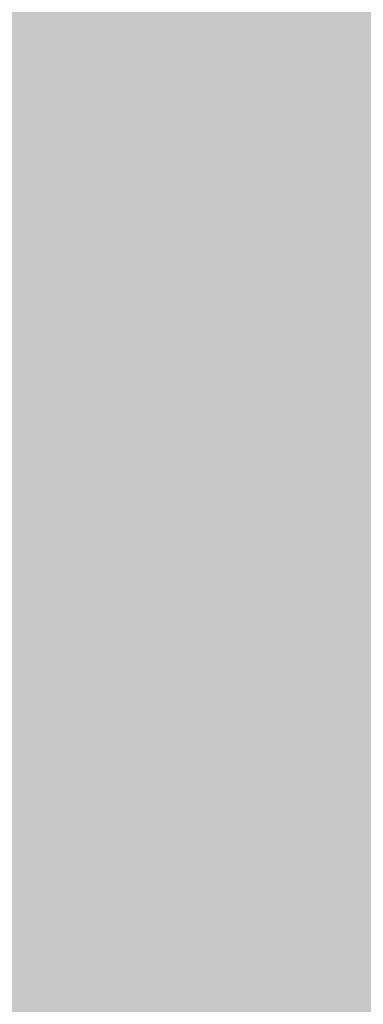
# Model space of a CAD drawing. Units: inches. Extents: x 2091 to 2899, y 967 to 2217.
# Tile 255 of 256: x 2246.06 to 2253.52, y 1131.25 to 1152.59. Entities that reach past the tile are written whole.
import ezdxf

# ---------------------------------------------------------------- set-up
doc = ezdxf.new("R2010")
doc.units = ezdxf.units.IN
doc.layers.add('A-ANNO-DIMS', color=2, linetype='Continuous', lineweight=18)
doc.layers.add('A-WALL-PATT', color=141, linetype='Continuous', lineweight=13, true_color=0xadddf7)
doc.layers.add('L-PLNT-PATT', color=114, linetype='Continuous', lineweight=13, true_color=0x139b48)
doc.styles.get("Standard").update_dxf_attribs({"font": 'arial.ttf'})
doc.dimstyles.new('ISO-25', dxfattribs={"dimtxt": 4, "dimasz": 4, "dimexe": 1.25, "dimexo": 0.625, "dimtad": 1, "dimdec": 0, "dimlunit": 3, "dimtxsty": 'Standard', "dimcen": 2.5, "dimadec": 0, "dimazin": 0, "dimtfac": 1, "dimtdec": 0, "dimtmove": 0, "dimatfit": 3, "dimfxl": 1, "dimarcsym": 0})

# ---------------------------------------------------------------- blocks, each defined once
blk = doc.blocks.new('*D71')
at = {"layer": 'A-ANNO-DIMS', "color": 0, "lineweight": -2, "transparency": 16777216}
for p, q in [((2212.144, 1351.294), (2212.144, 969.464)), ((2452.144, 1351.294), (2452.144, 969.464)), ((2216.144, 970.714), (2448.144, 970.714))]:
    blk.add_line(p, q, dxfattribs=at)
at = {"layer": 'A-ANNO-DIMS', "color": 0, "transparency": 16777216}
for points in [[(2216.144, 971.381), (2216.144, 970.048), (2212.144, 970.714)], [(2448.144, 971.381), (2448.144, 970.048), (2452.144, 970.714)]]:
    blk.add_solid(points, dxfattribs=at)
at = {"layer": 'Defpoints', "color": 0, "transparency": 16777216}
for p in [(2212.144, 1351.919), (2452.144, 1351.919), (2452.144, 970.714)]:
    blk.add_point(p, dxfattribs=at)
at = {"layer": 'A-ANNO-DIMS', "color": 0, "transparency": 16777216, "insert": (2332.144, 973.382), "char_height": 4, "attachment_point": 5}
blk.add_mtext('20\'-0"', dxfattribs=at)
blk = doc.blocks.new('*D75')
at = {"layer": 'A-ANNO-DIMS', "color": 0, "lineweight": -2, "transparency": 16777216}
for p, q in [((2212.144, 1274.794), (2212.144, 969.464)), ((2308.144, 1274.794), (2308.144, 969.464)), ((2216.144, 970.714), (2304.144, 970.714))]:
    blk.add_line(p, q, dxfattribs=at)
at = {"layer": 'A-ANNO-DIMS', "color": 0, "transparency": 16777216}
for points in [[(2216.144, 971.381), (2216.144, 970.048), (2212.144, 970.714)], [(2304.144, 971.381), (2304.144, 970.048), (2308.144, 970.714)]]:
    blk.add_solid(points, dxfattribs=at)
at = {"layer": 'Defpoints', "color": 0, "transparency": 16777216}
for p in [(2212.144, 1275.419), (2308.144, 1275.419), (2308.144, 970.714)]:
    blk.add_point(p, dxfattribs=at)
at = {"layer": 'A-ANNO-DIMS', "color": 0, "transparency": 16777216, "insert": (2260.144, 973.382), "char_height": 4, "attachment_point": 5}
blk.add_mtext('8\'-0"', dxfattribs=at)

msp = doc.modelspace()

# ---------------------------------------------------------------- hatches: boundary and pattern name
at = {"layer": 'A-WALL-PATT'}
h = msp.add_hatch(color=256, dxfattribs=at)
h.dxf.hatch_style = 1
h.paths.add_polyline_path([(2803.144, 2050.919), (2203.144, 2050.919), (2203.144, 1090.919), (2803.144, 1090.919)])
h.paths.add_polyline_path([(2635.799, 1147.54), (2674.524, 1147.54, 0.376086), (2678.53, 1152.88), (2678.53, 1159.556, 0.333335), (2674.524, 1163.562), (2674.524, 1163.562), (2674.524, 1192.934), (2635.806, 1192.934), (2597.088, 1192.934), (2597.088, 1163.562, 0.333335), (2593.082, 1159.556), (2593.082, 1152.88, 0.376086), (2597.088, 1147.54)], flags=0)
h.paths.add_polyline_path([(2436.01, 1278.241, 0.000483), (2435.953, 1278.215, -0.001328), (2435.936, 1278.112, -0.001711), (2436.116, 1278.041, 0.002185)], flags=0)
h.paths.add_polyline_path([(2794.144, 1143.419), (2794.144, 1347.419), (2543.37, 1347.419), (2543.37, 1351.919), (2794.144, 1351.919), (2794.144, 1392.714), (2793.947, 1392.714), (2793.947, 1473.537), (2794.144, 1473.537), (2794.144, 1531.919), (2650.144, 1531.919), (2650.144, 1536.419), (2794.144, 1536.419), (2794.144, 1692.419), (2609.376, 1692.419), (2609.376, 1644.419), (2604.876, 1644.419), (2604.876, 1744.919), (2609.376, 1744.919), (2609.376, 1696.919), (2794.144, 1696.919), (2794.144, 1780.919), (2609.644, 1780.919), (2493.876, 1780.919), (2493.876, 1785.419), (2609.644, 1785.419), (2794.144, 1785.419), (2794.144, 1847.939), (2793.951, 1847.939), (2793.951, 1928.762), (2794.144, 1928.762), (2794.144, 1941.419), (2614.144, 1941.419), (2614.144, 1821.419), (2609.644, 1821.419), (2609.644, 1941.419), (2392.144, 1941.419), (2392.144, 1819.919), (2387.644, 1819.919), (2387.644, 1941.419), (2212.144, 1941.419), (2212.144, 1783.919), (2392.144, 1783.919), (2392.144, 1780.919), (2212.144, 1780.919), (2212.144, 1629.419), (2387.644, 1629.419), (2387.644, 1744.919), (2392.144, 1744.919), (2392.144, 1627.919), (2317.144, 1627.919), (2317.144, 1551.419), (2317.144, 1536.419), (2459.384, 1536.419), (2459.384, 1602.396), (2463.884, 1602.396), (2463.884, 1531.919), (2456.644, 1531.919), (2456.644, 1529.919), (2452.144, 1529.919), (2452.144, 1531.919), (2312.644, 1531.919), (2312.644, 1551.419), (2306.144, 1551.419), (2306.144, 1555.919), (2308.144, 1555.919), (2308.144, 1551.419), (2312.644, 1551.419), (2312.644, 1627.919), (2212.144, 1627.919), (2212.144, 1555.919), (2270.144, 1555.919), (2270.144, 1551.419), (2212.144, 1551.419), (2212.144, 1351.919), (2272.144, 1351.919), (2272.144, 1347.419), (2212.144, 1347.419), (2212.144, 1275.419), (2308.144, 1275.419), (2308.144, 1351.919), (2452.144, 1351.919), (2452.144, 1493.919), (2456.644, 1493.919), (2456.644, 1347.419), (2312.644, 1347.419), (2312.644, 1270.919), (2212.144, 1270.919), (2212.144, 1099.919), (2281.238, 1099.919), (2282.871, 1110.914), (2282.008, 1116.997), (2278.558, 1121.42), (2268.206, 1128.056), (2272.088, 1128.056), (2273.813, 1131.927), (2279.42, 1134.692), (2285.028, 1135.245), (2287.616, 1137.457), (2288.047, 1138.01), (2289.341, 1140.775), (2291.067, 1139.669), (2292.361, 1135.245), (2295.38, 1136.904), (2296.243, 1135.798), (2297.105, 1133.033), (2300.125, 1138.01), (2303.144, 1138.01), (2304.438, 1135.798), (2303.144, 1133.586), (2306.595, 1134.692), (2307.889, 1133.033), (2310.908, 1135.245), (2313.927, 1134.139), (2315.627, 1132.427), (2308.32, 1117.55), (2290.204, 1109.808), (2288.91, 1103.172), (2289.272, 1099.919), (2434.918, 1099.919), (2431.593, 1124.788), (2429.93, 1169.553), (2430.927, 1240.52), (2435.659, 1238.186), (2437.135, 1196.554), (2438.798, 1143.973), (2442.678, 1111.998), (2446.558, 1099.919), (2794.144, 1099.919), (2794.144, 1138.919), (2548.032, 1138.919), (2548.032, 1143.419), (2548.032, 1148.819), (2546.668, 1148.032), (2528.686, 1179.179, 0.256256), (2512.032, 1148.819), (2512.032, 1143.419), (2512.032, 1138.919), (2507.532, 1138.919), (2507.532, 1143.419), (2507.532, 1148.819, 0.256256), (2490.879, 1179.179), (2472.896, 1148.032), (2471.532, 1148.819), (2471.532, 1143.419), (2467.032, 1143.419), (2467.032, 1269.946, 0.039061), (2460.91, 1273.58), (2467.032, 1273.58), (2467.032, 1286.325, 0.014511), (2465.216, 1286.762), (2467.032, 1287.053), (2467.032, 1323.419), (2471.532, 1323.419), (2471.532, 1148.819), (2489.532, 1179.996), (2490.896, 1179.208), (2490.879, 1179.179, -0.256256), (2507.532, 1148.819), (2507.532, 1143.419), (2512.032, 1143.419), (2512.032, 1148.819, -0.256256), (2528.686, 1179.179), (2528.668, 1179.208), (2530.032, 1179.996), (2548.032, 1148.819), (2548.032, 1143.419)], flags=16)
h.paths.add_polyline_path([(2607.769, 1200.945), (2607.769, 1265.031), (2597.088, 1281.052), (2619.785, 1281.052), (2627.795, 1337.127), (2635.799, 1337.127), (2643.817, 1337.127), (2651.827, 1281.052), (2674.524, 1281.052), (2663.843, 1265.031), (2663.843, 1200.945), (2635.806, 1200.945)], flags=0)
edge = h.paths.add_edge_path(flags=0)
edge.add_ellipse((13303.896, 1272.999), major_axis=(-10595.313, 0), ratio=0.84230387, start_angle=0.6282372, end_angle=0.6465541, ccw=False)
edge.add_ellipse((2711.7, 1156.853), major_axis=(2.22, 0), ratio=0.842304, start_angle=111.5352, end_angle=180.6282, ccw=False)
edge.add_ellipse((13303.156, 1272.999), major_axis=(-10593.026, 0), ratio=0.84230387, start_angle=0.5282715, end_angle=0.6465541, ccw=False)
edge.add_line((2710.765, 1175.333), (2710.13, 1175.333))
edge.add_ellipse((2710.13, 1176.58), major_axis=(1.48, 0), ratio=0.842304, start_angle=180, end_angle=270, ccw=False)
edge.add_line((2708.65, 1176.58), (2708.65, 1200.783))
edge.add_ellipse((2710.13, 1200.783), major_axis=(1.48, 0), ratio=0.842304, start_angle=90, end_angle=180, ccw=False)
edge.add_line((2710.13, 1202.029), (2710.465, 1202.029))
edge.add_ellipse((13303.156, 1272.999), major_axis=(-10593.026, 0), ratio=0.84230387, start_angle=-0.0902291, end_angle=0.3838668, ccw=False)
edge.add_ellipse((2710.13, 1290.927), major_axis=(-1.48, 0), ratio=0.842304, start_angle=0, end_angle=90, ccw=False)
edge.add_line((2708.65, 1290.927), (2708.65, 1315.13))
edge.add_ellipse((2710.13, 1315.13), major_axis=(-1.48, 0), ratio=0.842304, start_angle=-90, end_angle=0, ccw=False)
edge.add_line((2710.13, 1316.377), (2710.706, 1316.377))
edge.add_ellipse((3238.402, 1296.29), major_axis=(528.234, 0), ratio=0.8423039, start_angle=176.34957, end_angle=177.82005, ccw=False)
edge.add_ellipse((2775.063, 1071.451), major_axis=(313.308, 0), ratio=0.8423039, start_angle=102.12597, end_angle=103.78053, ccw=False)
edge.add_ellipse((2775.063, 1078.306), major_axis=(-305.303, 0), ratio=0.8423039, start_angle=-79.79046, end_angle=-77.55537, ccw=False)
edge.add_ellipse((2695.142, 1541.975), major_axis=(-250.96, 0), ratio=0.8423039, start_angle=99.25657, end_angle=102.55493)
edge.add_line((2741.41, 1334.214), (2747.133, 1337.378))
edge.add_ellipse((2747.539, 1336.857), major_axis=(-0.74, 0), ratio=0.842304, start_angle=270, end_angle=307.9331, ccw=False)
edge.add_ellipse((2747.539, 1336.857), major_axis=(-0.74, 0), ratio=0.842304, start_angle=232.0669, end_angle=270, ccw=False)
edge.add_line((2747.945, 1337.378), (2753.667, 1334.214))
edge.add_ellipse((2799.935, 1541.975), major_axis=(250.96, 0), ratio=0.8423039, start_angle=257.44507, end_angle=260.74343)
edge.add_ellipse((2720.014, 1078.306), major_axis=(305.303, 0), ratio=0.8423039, start_angle=77.55537, end_angle=79.79046, ccw=False)
edge.add_ellipse((2720.014, 1071.451), major_axis=(-313.308, 0), ratio=0.8423039, start_angle=256.21947, end_angle=257.87403, ccw=False)
edge.add_ellipse((2256.676, 1296.29), major_axis=(-528.234, 0), ratio=0.8423039, start_angle=182.17995, end_angle=183.65043, ccw=False)
edge.add_line((2784.371, 1316.377), (2784.947, 1316.377))
edge.add_ellipse((2784.947, 1315.13), major_axis=(1.48, 0), ratio=0.842304, start_angle=0, end_angle=90, ccw=False)
edge.add_line((2786.427, 1315.13), (2786.427, 1290.927))
edge.add_ellipse((2784.947, 1290.927), major_axis=(1.48, 0), ratio=0.842304, start_angle=270, end_angle=360, ccw=False)
edge.add_ellipse((-7808.079, 1272.999), major_axis=(10593.026, 0), ratio=0.84230387, start_angle=-0.3838668, end_angle=0.0902291, ccw=False)
edge.add_line((2784.612, 1202.029), (2784.947, 1202.029))
edge.add_ellipse((2784.947, 1200.783), major_axis=(1.48, 0), ratio=0.842304, start_angle=0, end_angle=90, ccw=False)
edge.add_line((2786.427, 1200.783), (2786.427, 1176.58))
edge.add_ellipse((2784.947, 1176.58), major_axis=(-1.48, 0), ratio=0.842304, start_angle=90, end_angle=180, ccw=False)
edge.add_line((2784.947, 1175.333), (2784.313, 1175.333))
edge.add_ellipse((-7808.079, 1272.999), major_axis=(10593.026, 0), ratio=0.84230387, start_angle=-0.6186432, end_angle=-0.5282715, ccw=False)
edge.add_ellipse((2783.377, 1156.853), major_axis=(-2.22, 0), ratio=0.842304, start_angle=179.3718, end_angle=248.4648, ccw=False)
edge.add_ellipse((-7808.819, 1272.999), major_axis=(-10595.313, 0), ratio=0.842303866, start_angle=179.3534459, end_angle=179.3717628, ccw=False)
edge.add_ellipse((2780.297, 1153.501), major_axis=(-5.246, 0), ratio=0.842304, start_angle=90, end_angle=179.3534, ccw=False)
edge.add_line((2780.297, 1149.082), (2714.78, 1149.082))
edge.add_ellipse((2714.78, 1153.501), major_axis=(5.246, 0), ratio=0.842304, start_angle=180.6466, end_angle=270, ccw=False)
edge = h.paths.add_edge_path(flags=0)
edge.add_line((2718.187, 1151.008), (2718.187, 1170.472))
edge.add_ellipse((2721.147, 1170.472), major_axis=(-2.96, 0), ratio=0.842304, start_angle=-90, end_angle=0, ccw=False)
edge.add_line((2721.147, 1172.965), (2773.93, 1172.965))
edge.add_ellipse((2773.93, 1170.472), major_axis=(-2.96, 0), ratio=0.842304, start_angle=180, end_angle=270, ccw=False)
edge.add_line((2776.89, 1170.472), (2776.89, 1151.008))
edge.add_line((2776.89, 1151.008), (2718.187, 1151.008))
edge = h.paths.add_edge_path(flags=0)
edge.add_line((2718.187, 1180.234), (2718.187, 1199.058))
edge.add_ellipse((2747.539, 1320.399), major_axis=(147.018, 0), ratio=0.8423039, start_angle=256.40187, end_angle=283.59813)
edge.add_line((2776.89, 1199.058), (2776.89, 1180.234))
edge.add_ellipse((2747.539, 1301.575), major_axis=(147.018, 0), ratio=0.8423039, start_angle=256.40187, end_angle=283.59813, ccw=False)
edge = h.paths.add_edge_path(flags=0)
edge.add_ellipse((13303.156, 1272.999), major_axis=(-10591.546, 0), ratio=0.84230387, start_angle=0.0555943, end_angle=0.3777642, ccw=False)
edge.add_line((2711.617, 1262.722), (2715.667, 1249.495))
edge.add_ellipse((6413.892, 1241.692), major_axis=(-3698.236, 0), ratio=0.84230387, start_angle=-0.120897, end_angle=0.364076)
edge.add_line((2715.761, 1218.192), (2711.934, 1203.167))
edge = h.paths.add_edge_path(flags=0)
edge.add_line((2718.187, 1251.075), (2716.002, 1267.45))
edge.add_ellipse((2742.151, 1202.19), major_axis=(81.773, 0), ratio=0.842304, start_angle=94.27742, end_angle=111.83495, ccw=False)
edge.add_line((2737.01, 1270.931), (2758.067, 1270.931))
edge.add_ellipse((2752.926, 1202.19), major_axis=(81.773, 0), ratio=0.842304, start_angle=68.16505, end_angle=85.72258, ccw=False)
edge.add_line((2779.075, 1267.45), (2776.89, 1251.075))
edge.add_ellipse((2750.338, 1187.885), major_axis=(79.58, 0), ratio=0.842304, start_angle=67.20809, end_angle=85.12993)
edge.add_line((2756.035, 1254.744), (2739.043, 1254.744))
edge.add_ellipse((2744.739, 1187.885), major_axis=(79.58, 0), ratio=0.842304, start_angle=94.87007, end_angle=112.79191)
edge = h.paths.add_edge_path(flags=0)
edge.add_line((2783.143, 1203.167), (2779.316, 1218.192))
edge.add_ellipse((-918.815, 1241.692), major_axis=(3698.236, 0), ratio=0.84230387, start_angle=-0.364076, end_angle=0.120897)
edge.add_line((2779.41, 1249.495), (2783.46, 1262.722))
edge.add_ellipse((-7808.079, 1272.999), major_axis=(-10591.546, 0), ratio=0.84230387, start_angle=179.6222358, end_angle=179.9444057, ccw=False)
edge = h.paths.add_edge_path(flags=0)
edge.add_ellipse((2734.201, 1286.69), major_axis=(-0.357, 6.34), ratio=0.603834, start_angle=89.002, end_angle=253.6574, ccw=False)
edge.add_line((2730.369, 1286.542), (2730.369, 1301.352))
edge.add_line((2730.369, 1301.352), (2735.913, 1305.215))
edge.add_ellipse((2736.385, 1304.735), major_axis=(0.74, 0), ratio=0.842304, start_angle=90, end_angle=134.4802, ccw=False)
edge.add_line((2736.385, 1305.358), (2738.033, 1305.358))
edge.add_line((2738.033, 1305.358), (2738.033, 1307.708))
edge.add_ellipse((2794.202, 1307.708), major_axis=(56.169, 0), ratio=0.842304, start_angle=150.5614, end_angle=180, ccw=False)
edge.add_ellipse((2700.876, 1307.708), major_axis=(-56.169, 0), ratio=0.842304, start_angle=180, end_angle=209.4386, ccw=False)
edge.add_line((2757.044, 1307.708), (2757.044, 1305.358))
edge.add_line((2757.044, 1305.358), (2758.692, 1305.358))
edge.add_ellipse((2758.692, 1304.735), major_axis=(-0.74, 0), ratio=0.842304, start_angle=225.5198, end_angle=270, ccw=False)
edge.add_line((2759.164, 1305.215), (2764.708, 1301.352))
edge.add_line((2764.708, 1301.352), (2764.708, 1286.542))
edge.add_ellipse((2760.876, 1286.69), major_axis=(0.357, 6.34), ratio=0.603834, start_angle=106.3426, end_angle=270.998, ccw=False)
edge.add_line((2757.044, 1285.797), (2757.044, 1307.708))
edge.add_ellipse((2700.876, 1307.708), major_axis=(-56.169, 0), ratio=0.842304, start_angle=180, end_angle=209.4386)
edge.add_ellipse((2794.202, 1307.708), major_axis=(56.169, 0), ratio=0.842304, start_angle=150.5614, end_angle=180)
edge.add_line((2738.033, 1307.708), (2738.033, 1285.797))
h.paths.add_polyline_path([(2417.812, 1104.45), (2413.492, 1102.53), (2410.612, 1103.97), (2409.172, 1106.37), (2407.252, 1107.33), (2406.292, 1109.73), (2405.332, 1114.05), (2405.332, 1117.89), (2406.292, 1120.13), (2407.252, 1119.81), (2408.848, 1118.328), (2410.174, 1119.424), (2410.211, 1120.406), (2411.041, 1121.419), (2410.699, 1119.859), (2410.174, 1119.424), (2410.088, 1117.176), (2411.133, 1116.206), (2413.972, 1119.33), (2416.852, 1120.77), (2416.87, 1120.799), (2417.035, 1119.405), (2417.896, 1118.143), (2418.292, 1118.37), (2419.544, 1120.039), (2419.361, 1118.387), (2419.032, 1119.356), (2418.399, 1118.512), (2419.252, 1114.53), (2418.794, 1107.199)], flags=0)
h.paths.add_polyline_path([(2508.87, 1347.419), (2508.37, 1347.419), (2508.37, 1351.919), (2508.87, 1351.919)], flags=0)
h.paths.add_polyline_path([(2473.37, 1347.419), (2472.37, 1347.419), (2467.87, 1347.419), (2467.87, 1455.419), (2472.37, 1455.419), (2472.37, 1352.419), (2473.37, 1352.419)], flags=0)
h.paths.add_polyline_path([(2352.106, 1217.446), (2349.226, 1218.886), (2347.786, 1221.286), (2345.866, 1222.246), (2344.906, 1224.646), (2343.946, 1228.966), (2343.946, 1232.806), (2344.906, 1235.046), (2345.866, 1234.726), (2347.462, 1233.244), (2348.788, 1234.341), (2348.825, 1235.322), (2349.655, 1236.336), (2349.313, 1234.775), (2348.788, 1234.341), (2348.702, 1232.093), (2349.747, 1231.123), (2352.586, 1234.246), (2355.466, 1235.686), (2355.484, 1235.715), (2355.649, 1234.322), (2356.51, 1233.06), (2356.906, 1233.286), (2358.158, 1234.956), (2357.975, 1233.304), (2357.646, 1234.273), (2357.013, 1233.428), (2357.866, 1229.446), (2357.408, 1222.115), (2356.426, 1219.366)], flags=0)
h.paths.add_polyline_path([(2348.297, 1112.224), (2347.014, 1112.31), (2345.53, 1114.127), (2345.732, 1115.858), (2346.812, 1116.982), (2346.812, 1114.646), (2345.867, 1114.214), (2346.88, 1114.3)], flags=0)
h.paths.add_polyline_path([(2347.014, 1110.926), (2346.272, 1110.493), (2346.61, 1111.186)], flags=0)
h.paths.add_polyline_path([(2345.867, 1118.194), (2345.53, 1117.329), (2343.708, 1118.021), (2344.383, 1118.626)], flags=0)
h.paths.add_polyline_path([(2346.677, 1109.282), (2346.07, 1108.071), (2345.867, 1110.061)], flags=0)
h.paths.add_polyline_path([(2345.057, 1119.751), (2343.64, 1119.751), (2343.978, 1121.135)], flags=0)
h.paths.add_polyline_path([(2345.26, 1116.55), (2345.125, 1115.858), (2344.922, 1115.685), (2344.72, 1116.377)], flags=0)
h.paths.add_polyline_path([(2345.665, 1112.31), (2345.462, 1111.532), (2344.045, 1111.964), (2344.652, 1112.57)], flags=0)
h.paths.add_polyline_path([(2345.192, 1113.349), (2344.45, 1113.868), (2344.72, 1114.387)], flags=0)
h.paths.add_polyline_path([(2344.652, 1116.809), (2344.18, 1115.685), (2344.652, 1115.339), (2343.91, 1114.906), (2343.033, 1115.944), (2343.64, 1116.463)], flags=0)
h.paths.add_polyline_path([(2345.867, 1106.686), (2344.99, 1105.562), (2344.517, 1106.6)], flags=0)
h.paths.add_polyline_path([(2344.855, 1110.061), (2344.517, 1109.282), (2344.113, 1109.715)], flags=0)
h.paths.add_polyline_path([(2344.045, 1113.522), (2343.438, 1113.089), (2342.763, 1113.954)], flags=0)
h.paths.add_polyline_path([(2344.315, 1111.012), (2342.965, 1110.32), (2342.965, 1111.099)], flags=0)
h.paths.add_polyline_path([(2345.125, 1104.697), (2344.585, 1103.745), (2344.45, 1104.264)], flags=0)
h.paths.add_polyline_path([(2342.83, 1121.222), (2341.75, 1120.53), (2340.536, 1121.049), (2340.131, 1121.828), (2340.671, 1122.952), (2341.143, 1121.828), (2341.615, 1122.001)], flags=0)
h.paths.add_polyline_path([(2342.965, 1119.751), (2343.033, 1118.453), (2342.088, 1118.021), (2342.02, 1119.491)], flags=0)
h.paths.add_polyline_path([(2342.695, 1116.896), (2341.953, 1116.636), (2342.02, 1117.329)], flags=0)
h.paths.add_polyline_path([(2343.033, 1112.224), (2342.02, 1111.791), (2341.548, 1112.224), (2342.358, 1113.349)], flags=0)
h.paths.add_polyline_path([(2343.775, 1104.437), (2342.628, 1102.88), (2342.695, 1104.61), (2343.438, 1105.129)], flags=0)
h.paths.add_polyline_path([(2342.02, 1115.079), (2340.806, 1115.512), (2340.941, 1116.377)], flags=0)
h.paths.add_polyline_path([(2341.481, 1120.097), (2341.481, 1119.405), (2341.076, 1119.578), (2341.143, 1120.097)], flags=0)
h.paths.add_polyline_path([(2341.818, 1114.473), (2340.941, 1113.089), (2340.806, 1114.56)], flags=0)
h.paths.add_polyline_path([(2341.143, 1118.54), (2340.941, 1116.982), (2339.051, 1117.675), (2339.051, 1118.626)], flags=0)
h.paths.add_polyline_path([(2342.695, 1101.668), (2341.953, 1101.841), (2342.56, 1102.361)], flags=0)
h.paths.add_polyline_path([(2340.333, 1119.665), (2338.444, 1119.578), (2337.904, 1120.357), (2339.658, 1120.616)], flags=0)
h.paths.add_polyline_path([(2340.333, 1115.339), (2340.063, 1113.695), (2339.388, 1115.339)], flags=0)
h.paths.add_polyline_path([(2341.818, 1103.831), (2341.548, 1102.88), (2341.143, 1103.658)], flags=0)
h.paths.add_polyline_path([(2339.051, 1122.866), (2337.296, 1121.828), (2337.094, 1123.125), (2337.769, 1123.818)], flags=0)
h.paths.add_polyline_path([(2339.118, 1121.741), (2338.848, 1121.222), (2338.174, 1121.049), (2338.376, 1121.568)], flags=0)
h.paths.add_polyline_path([(2339.186, 1119.319), (2338.646, 1118.713), (2338.241, 1118.107), (2338.241, 1118.886)], flags=0)
h.paths.add_polyline_path([(2341.143, 1101.928), (2340.603, 1101.236), (2340.063, 1101.841), (2340.603, 1102.361)], flags=0)
h.paths.add_polyline_path([(2337.634, 1117.761), (2336.621, 1118.28), (2337.296, 1118.972)], flags=0)
h.paths.add_polyline_path([(2336.824, 1119.578), (2334.799, 1118.972), (2335.204, 1120.357), (2336.554, 1120.876)], flags=0)
h.paths.add_polyline_path([(2339.118, 1100.457), (2337.364, 1100.543), (2336.756, 1101.236)], flags=0)
h.paths.add_polyline_path([(2336.351, 1122.433), (2336.014, 1121.914), (2334.934, 1122.433), (2334.529, 1123.471), (2335.744, 1122.779)], flags=0)
h.paths.add_polyline_path([(2334.732, 1120.876), (2334.259, 1120.357), (2334.057, 1120.789), (2334.597, 1121.308)], flags=0)
h.paths.add_polyline_path([(2334.462, 1122.174), (2332.572, 1121.308), (2331.357, 1122.174), (2332.1, 1122.866)], flags=0)
h.paths.add_polyline_path([(2334.259, 1118.54), (2333.382, 1118.453), (2333.652, 1119.319)], flags=0)
h.paths.add_polyline_path([(2335.542, 1102.274), (2334.192, 1102.62), (2335.272, 1103.312)], flags=0)
h.paths.add_polyline_path([(2332.707, 1119.665), (2331.695, 1120.443), (2332.505, 1120.789)], flags=0)
h.paths.add_polyline_path([(2334.732, 1101.149), (2333.517, 1101.582), (2333.989, 1101.755)], flags=0)
h.paths.add_polyline_path([(2332.64, 1116.636), (2331.087, 1116.29), (2331.965, 1118.194)], flags=0)
h.paths.add_polyline_path([(2330.75, 1121.568), (2330.277, 1120.27), (2328.523, 1119.319), (2328.995, 1121.049)], flags=0)
h.paths.add_polyline_path([(2330.75, 1118.626), (2330.008, 1117.502), (2329.873, 1118.021)], flags=0)
h.paths.add_polyline_path([(2332.1, 1102.361), (2330.547, 1102.014), (2331.695, 1102.966)], flags=0)
h.paths.add_polyline_path([(2329.535, 1113.608), (2329.063, 1112.31), (2328.59, 1113.349)], flags=0)
h.paths.add_polyline_path([(2328.388, 1117.848), (2327.51, 1116.55), (2327.173, 1117.761)], flags=0)
h.paths.add_polyline_path([(2329.738, 1106.513), (2329.535, 1105.302), (2328.253, 1106.081)], flags=0)
h.paths.add_polyline_path([(2328.658, 1114.387), (2328.05, 1114.127), (2328.32, 1114.906)], flags=0)
h.paths.add_polyline_path([(2328.32, 1112.224), (2327.106, 1112.137), (2326.701, 1112.656)], flags=0)
h.paths.add_polyline_path([(2326.903, 1115.252), (2326.701, 1114.127), (2325.216, 1113.608), (2326.093, 1115.339)], flags=0)
h.paths.add_polyline_path([(2326.633, 1108.33), (2326.093, 1107.379), (2325.891, 1108.503), (2326.498, 1109.109)], flags=0)
h.paths.add_polyline_path([(2615.144, 1531.919), (2609.644, 1531.919), (2609.644, 1620.419), (2614.144, 1620.419), (2614.144, 1536.419), (2615.144, 1536.419)], flags=0)
h.paths.add_polyline_path([(2545.144, 1563.419), (2464.144, 1563.419), (2464.144, 1632.419), (2509.144, 1632.419), (2509.144, 1627.919), (2509.144, 1603.919), (2468.644, 1603.919), (2468.644, 1567.919), (2540.644, 1567.919), (2540.644, 1591.919), (2545.144, 1591.919)], flags=0)
h.paths.add_polyline_path([(2388.969, 1549.986), (2357.434, 1549.986), (2357.434, 1623.361), (2399.363, 1623.361), (2435.689, 1623.361), (2435.593, 1602.559), (2435.593, 1602.396), (2388.969, 1602.396)], flags=0)
h.paths.add_polyline_path([(2388.881, 1555.809), (2374.904, 1555.809), (2374.904, 1600.572), (2374.904, 1615.458), (2406.351, 1615.458), (2406.351, 1618.939), (2412.174, 1615.458), (2406.351, 1611.976), (2406.351, 1615.458), (2388.881, 1615.458)], flags=0)
h.paths.add_polyline_path([(2568.876, 1644.419), (2453.376, 1644.419), (2453.376, 1785.419), (2457.876, 1785.419), (2457.876, 1648.919), (2568.876, 1648.919)], flags=0)
h.paths.add_polyline_path([(2212.144, 1945.919), (2212.144, 2041.919), (2794.144, 2041.919), (2794.144, 1945.919)], flags=16)
h.paths.add_polyline_path([(2271.083, 1964.317), (2776.853, 1964.317), (2776.853, 2037.17), (2271.083, 2037.17)], flags=8)
h.paths.add_polyline_path([(2380.649, 1536.824), (2461.041, 1536.824), (2461.041, 1554.653), (2380.649, 1554.653)], flags=8)
h.paths.add_polyline_path([(2240.756, 1609.725), (2309.186, 1609.725), (2309.186, 1617.698), (2240.756, 1617.698)], flags=8)
h.paths.add_polyline_path([(2212.677, 1313.504), (2282.592, 1313.504), (2282.592, 1322.745), (2212.677, 1322.745)], flags=8)
h.paths.add_polyline_path([(2457.112, 1114.779), (2558.482, 1114.779), (2558.482, 1142.22), (2457.112, 1142.22)], flags=8)
h.paths.add_polyline_path([(2473.442, 1273.01), (2604.641, 1273.01), (2604.641, 1318.347), (2473.442, 1318.347)], flags=8)
h.paths.add_polyline_path([(2638.876, 1626.977), (2684.25, 1627.977), (2684.038, 1637.597), (2638.664, 1636.598)], flags=8)
h.paths.add_polyline_path([(2537.591, 1453.793), (2628.39, 1453.793), (2628.39, 1475.345), (2537.591, 1475.345)], flags=8)
h.paths.add_polyline_path([(2504.138, 1714.632), (2554.647, 1714.632), (2554.647, 1730.238), (2504.138, 1730.238)], flags=8)
h.paths.add_polyline_path([(2487.501, 1575.652), (2535.097, 1575.652), (2535.097, 1598.378), (2487.501, 1598.378)], flags=8)
h.paths.add_polyline_path([(2709.099, 1735.71), (2740.017, 1735.71), (2740.017, 1749.938), (2709.099, 1749.938)], flags=8)
h.paths.add_polyline_path([(2442.438, 1792.172), (2564.729, 1792.172), (2564.729, 1842), (2442.438, 1842)], flags=8)
h.paths.add_polyline_path([(2655.816, 1809.644), (2789.52, 1806.694), (2790.085, 1832.292), (2656.381, 1835.242)], flags=8)
h.paths.add_polyline_path([(2234.843, 1797.72), (2368.593, 1794.769), (2369.161, 1820.504), (2235.411, 1823.455)], flags=8)
h.paths.add_polyline_path([(2245.138, 1644.006), (2398.428, 1640.624), (2398.995, 1666.325), (2245.706, 1669.707)], flags=8)
h.paths.add_polyline_path([(2306.143, 1431.169), (2413.768, 1428.794), (2414.333, 1454.392), (2306.708, 1456.766)], flags=8)
h.paths.add_polyline_path([(2306.835, 1458.233), (2393.38, 1456.323), (2393.933, 1481.354), (2307.387, 1483.264)], flags=8)
at = {"layer": 'L-PLNT-PATT'}
h = msp.add_hatch(color=256, dxfattribs=at)
h.dxf.hatch_style = 1
h.paths.add_polyline_path([(2333.338, 1165.659), (2329.024, 1166.212), (2331.612, 1168.424), (2335.063, 1177.271), (2328.162, 1184.46), (2319.535, 1187.225), (2323.417, 1193.308), (2319.966, 1203.814), (2317.809, 1203.814), (2313.496, 1213.215), (2310.908, 1212.662), (2307.889, 1212.662), (2305.732, 1217.086), (2307.026, 1223.168), (2310.477, 1223.168), (2304.007, 1230.91), (2303.136, 1237.046), (2299.693, 1240.864), (2296.674, 1237.546), (2294.949, 1238.652), (2294.517, 1241.417), (2292.361, 1242.523), (2289.341, 1239.758), (2285.89, 1240.311), (2283.302, 1235.334), (2283.302, 1230.91), (2286.753, 1229.251), (2284.165, 1227.592), (2281.577, 1229.804), (2274.244, 1222.615), (2274.244, 1220.957), (2271.225, 1219.298), (2272.088, 1217.639), (2274.244, 1214.321), (2270.362, 1211.556), (2266.48, 1214.321), (2264.324, 1213.768), (2263.461, 1211.556), (2266.48, 1211.003), (2266.912, 1206.579), (2263.539, 1207.132), (2259.579, 1203.261), (2263.892, 1202.708), (2262.167, 1197.178), (2258.285, 1196.625), (2253.971, 1193.861), (2248.795, 1191.096), (2248.364, 1193.308), (2244.482, 1185.013), (2251.383, 1186.672), (2255.697, 1183.907), (2254.403, 1177.271), (2246.639, 1174.506), (2243.188, 1176.718), (2241.894, 1173.4), (2238.875, 1172.847), (2236.287, 1169.53), (2233.267, 1165.659), (2237.149, 1162.341), (2239.737, 1164), (2236.811, 1159.191), (2238.937, 1159.439), (2238.63, 1155.086), (2231.542, 1145.752), (2222.915, 1145.199), (2219.033, 1142.987), (2212.563, 1135.798), (2215.151, 1131.374), (2231.111, 1131.927), (2234.13, 1129.715), (2241.463, 1133.033), (2246.639, 1121.973), (2248.795, 1121.973), (2258.716, 1134.139), (2261.736, 1135.798), (2263.892, 1133.033), (2263.892, 1129.162), (2267.343, 1128.056), (2272.088, 1128.056), (2273.813, 1131.927), (2279.42, 1134.692), (2285.028, 1135.245), (2287.616, 1137.457), (2288.047, 1138.01), (2289.341, 1140.775), (2291.067, 1139.669), (2292.361, 1135.245), (2295.38, 1136.904), (2296.243, 1135.798), (2297.105, 1133.033), (2300.125, 1138.01), (2303.144, 1138.01), (2304.438, 1135.798), (2303.144, 1133.586), (2306.595, 1134.692), (2307.889, 1133.033), (2310.908, 1135.245), (2313.927, 1134.139), (2319.966, 1128.056), (2322.554, 1126.95), (2324.711, 1124.738), (2342.827, 1126.397), (2346.278, 1123.079), (2348.866, 1124.185), (2341.964, 1133.033), (2341.533, 1136.351), (2343.69, 1139.669), (2339.808, 1150.175), (2337.651, 1150.175)])
h.paths.add_polyline_path([(2339.658, 1120.616), (2337.904, 1120.357), (2338.444, 1119.578), (2340.333, 1119.665)])
h.paths.add_polyline_path([(2341.143, 1118.54), (2339.051, 1118.626), (2339.051, 1117.675), (2340.941, 1116.982)])
h.paths.add_polyline_path([(2336.554, 1120.876), (2335.204, 1120.357), (2334.799, 1118.972), (2336.824, 1119.578)])
h.paths.add_polyline_path([(2337.296, 1118.972), (2336.621, 1118.28), (2337.634, 1117.761)])
h.paths.add_polyline_path([(2338.646, 1118.713), (2339.186, 1119.319), (2338.241, 1118.886), (2338.241, 1118.107)])
h.paths.add_polyline_path([(2339.051, 1122.866), (2337.769, 1123.818), (2337.094, 1123.125), (2337.296, 1121.828)])
h.paths.add_polyline_path([(2341.615, 1122.001), (2341.143, 1121.828), (2340.671, 1122.952), (2340.131, 1121.828), (2340.536, 1121.049), (2341.75, 1120.53), (2342.83, 1121.222)])
h.paths.add_polyline_path([(2342.965, 1119.751), (2342.02, 1119.491), (2342.088, 1118.021), (2343.033, 1118.453)])
h.paths.add_polyline_path([(2345.867, 1118.194), (2344.383, 1118.626), (2343.708, 1118.021), (2345.53, 1117.329)])
h.paths.add_polyline_path([(2344.652, 1116.809), (2343.64, 1116.463), (2343.033, 1115.944), (2343.91, 1114.906), (2344.652, 1115.339), (2344.18, 1115.685)])
h.paths.add_polyline_path([(2346.812, 1116.982), (2345.732, 1115.858), (2345.53, 1114.127), (2347.014, 1112.31), (2348.297, 1112.224), (2346.88, 1114.3), (2345.867, 1114.214), (2346.812, 1114.646)])
h.paths.add_polyline_path([(2345.26, 1116.55), (2344.72, 1116.377), (2344.922, 1115.685), (2345.125, 1115.858)])
h.paths.add_polyline_path([(2342.695, 1116.896), (2342.02, 1117.329), (2341.953, 1116.636)])
h.paths.add_polyline_path([(2341.481, 1120.097), (2341.143, 1120.097), (2341.076, 1119.578), (2341.481, 1119.405)])
h.paths.add_polyline_path([(2343.978, 1121.135), (2343.64, 1119.751), (2345.057, 1119.751)])
h.paths.add_polyline_path([(2339.118, 1121.741), (2338.376, 1121.568), (2338.174, 1121.049), (2338.848, 1121.222)])
h.paths.add_polyline_path([(2336.351, 1122.433), (2335.744, 1122.779), (2334.529, 1123.471), (2334.934, 1122.433), (2336.014, 1121.914)])
h.paths.add_polyline_path([(2334.462, 1122.174), (2332.1, 1122.866), (2331.357, 1122.174), (2332.572, 1121.308)])
h.paths.add_polyline_path([(2334.597, 1121.308), (2334.057, 1120.789), (2334.259, 1120.357), (2334.732, 1120.876)])
h.paths.add_polyline_path([(2332.505, 1120.789), (2331.695, 1120.443), (2332.707, 1119.665)])
h.paths.add_polyline_path([(2333.652, 1119.319), (2333.382, 1118.453), (2334.259, 1118.54)])
h.paths.add_polyline_path([(2331.965, 1118.194), (2331.087, 1116.29), (2332.64, 1116.636)])
h.paths.add_polyline_path([(2330.75, 1121.568), (2328.995, 1121.049), (2328.523, 1119.319), (2330.277, 1120.27)])
h.paths.add_polyline_path([(2330.75, 1118.626), (2329.873, 1118.021), (2330.008, 1117.502)])
h.paths.add_polyline_path([(2328.388, 1117.848), (2327.173, 1117.761), (2327.51, 1116.55)])
h.paths.add_polyline_path([(2326.903, 1115.252), (2326.093, 1115.339), (2325.216, 1113.608), (2326.701, 1114.127)])
h.paths.add_polyline_path([(2328.658, 1114.387), (2328.32, 1114.906), (2328.05, 1114.127)])
h.paths.add_polyline_path([(2326.701, 1112.656), (2327.106, 1112.137), (2328.32, 1112.224)])
h.paths.add_polyline_path([(2329.535, 1113.608), (2328.59, 1113.349), (2329.063, 1112.31)])
h.paths.add_polyline_path([(2340.333, 1115.339), (2339.388, 1115.339), (2340.063, 1113.695)])
h.paths.add_polyline_path([(2340.941, 1116.377), (2340.806, 1115.512), (2342.02, 1115.079)])
h.paths.add_polyline_path([(2341.818, 1114.473), (2340.806, 1114.56), (2340.941, 1113.089)])
h.paths.add_polyline_path([(2343.033, 1112.224), (2342.358, 1113.349), (2341.548, 1112.224), (2342.02, 1111.791)])
h.paths.add_polyline_path([(2342.763, 1113.954), (2343.438, 1113.089), (2344.045, 1113.522)])
h.paths.add_polyline_path([(2344.72, 1114.387), (2344.45, 1113.868), (2345.192, 1113.349)])
h.paths.add_polyline_path([(2345.665, 1112.31), (2344.652, 1112.57), (2344.045, 1111.964), (2345.462, 1111.532)])
h.paths.add_polyline_path([(2344.315, 1111.012), (2342.965, 1111.099), (2342.965, 1110.32)])
h.paths.add_polyline_path([(2344.855, 1110.061), (2344.113, 1109.715), (2344.517, 1109.282)])
h.paths.add_polyline_path([(2346.677, 1109.282), (2345.867, 1110.061), (2346.07, 1108.071)])
h.paths.add_polyline_path([(2347.014, 1110.926), (2346.61, 1111.186), (2346.272, 1110.493)])
h.paths.add_polyline_path([(2345.867, 1106.686), (2344.517, 1106.6), (2344.99, 1105.562)])
h.paths.add_polyline_path([(2345.125, 1104.697), (2344.45, 1104.264), (2344.585, 1103.745)])
h.paths.add_polyline_path([(2343.775, 1104.437), (2343.438, 1105.129), (2342.695, 1104.61), (2342.628, 1102.88)])
h.paths.add_polyline_path([(2341.818, 1103.831), (2341.143, 1103.658), (2341.548, 1102.88)])
h.paths.add_polyline_path([(2342.56, 1102.361), (2341.953, 1101.841), (2342.695, 1101.668)])
h.paths.add_polyline_path([(2341.143, 1101.928), (2340.603, 1102.361), (2340.063, 1101.841), (2340.603, 1101.236)])
h.paths.add_polyline_path([(2336.756, 1101.236), (2337.364, 1100.543), (2339.118, 1100.457)])
h.paths.add_polyline_path([(2335.272, 1103.312), (2334.192, 1102.62), (2335.542, 1102.274)])
h.paths.add_polyline_path([(2333.989, 1101.755), (2333.517, 1101.582), (2334.732, 1101.149)])
h.paths.add_polyline_path([(2331.695, 1102.966), (2330.547, 1102.014), (2332.1, 1102.361)])
h.paths.add_polyline_path([(2329.738, 1106.513), (2328.253, 1106.081), (2329.535, 1105.302)])
h.paths.add_polyline_path([(2326.633, 1108.33), (2326.498, 1109.109), (2325.891, 1108.503), (2326.093, 1107.379)])
h.paths.add_polyline_path([(2240.596, 1257.814), (2239.584, 1257.468), (2238.977, 1256.949), (2239.854, 1255.911), (2240.596, 1256.344), (2240.124, 1256.69)])
h.paths.add_polyline_path([(2241.811, 1259.199), (2240.327, 1259.631), (2239.652, 1259.026), (2241.474, 1258.334)])
h.paths.add_polyline_path([(2242.756, 1257.987), (2241.676, 1256.863), (2241.474, 1255.132), (2242.958, 1253.315), (2244.241, 1253.229), (2242.824, 1255.305), (2241.811, 1255.219), (2242.756, 1255.651)])
h.paths.add_polyline_path([(2241.609, 1253.315), (2240.596, 1253.575), (2239.989, 1252.969), (2241.406, 1252.537)])
h.paths.add_polyline_path([(2240.664, 1255.392), (2240.394, 1254.873), (2241.136, 1254.354)])
h.paths.add_polyline_path([(2242.958, 1251.931), (2242.554, 1252.191), (2242.216, 1251.498)])
h.paths.add_polyline_path([(2240.259, 1252.017), (2238.909, 1252.104), (2238.909, 1251.325)])
h.paths.add_polyline_path([(2238.302, 1254.354), (2237.492, 1253.229), (2237.964, 1252.796), (2238.977, 1253.229)])
h.paths.add_polyline_path([(2239.989, 1254.527), (2238.707, 1254.959), (2239.382, 1254.094)])
h.paths.add_polyline_path([(2240.799, 1251.066), (2240.057, 1250.72), (2240.461, 1250.287)])
h.paths.add_polyline_path([(2241.811, 1251.066), (2242.014, 1249.076), (2242.621, 1250.287)])
h.paths.add_polyline_path([(2241.204, 1257.555), (2240.664, 1257.382), (2240.866, 1256.69), (2241.069, 1256.863)])
h.paths.add_polyline_path([(2238.639, 1257.901), (2237.964, 1258.334), (2237.897, 1257.641)])
h.paths.add_polyline_path([(2238.909, 1260.756), (2237.964, 1260.496), (2238.032, 1259.026), (2238.977, 1259.458)])
h.paths.add_polyline_path([(2239.922, 1262.14), (2239.584, 1260.756), (2241.001, 1260.756)])
h.paths.add_polyline_path([(2238.774, 1262.227), (2237.559, 1263.006), (2237.087, 1262.833), (2236.615, 1263.957), (2236.075, 1262.833), (2236.48, 1262.054), (2237.694, 1261.535)])
h.paths.add_polyline_path([(2237.425, 1261.102), (2237.087, 1261.102), (2237.02, 1260.583), (2237.425, 1260.41)])
h.paths.add_polyline_path([(2237.087, 1259.545), (2234.995, 1259.631), (2234.995, 1258.68), (2236.885, 1257.987)])
h.paths.add_polyline_path([(2236.885, 1257.382), (2236.75, 1256.517), (2237.964, 1256.084)])
h.paths.add_polyline_path([(2237.762, 1255.478), (2236.75, 1255.565), (2236.885, 1254.094)])
h.paths.add_polyline_path([(2236.277, 1256.344), (2235.332, 1256.344), (2236.007, 1254.7)])
h.paths.add_polyline_path([(2241.811, 1247.691), (2240.461, 1247.605), (2240.934, 1246.567)])
h.paths.add_polyline_path([(2239.719, 1245.442), (2239.382, 1246.134), (2238.639, 1245.615), (2238.572, 1243.885)])
h.paths.add_polyline_path([(2241.069, 1245.702), (2240.394, 1245.269), (2240.529, 1244.75)])
h.paths.add_polyline_path([(2237.762, 1244.836), (2237.087, 1244.663), (2237.492, 1243.885)])
h.paths.add_polyline_path([(2237.087, 1242.933), (2236.547, 1243.366), (2236.007, 1242.846), (2236.547, 1242.241)])
h.paths.add_polyline_path([(2238.504, 1243.366), (2237.897, 1242.846), (2238.639, 1242.673)])
h.paths.add_polyline_path([(2232.7, 1242.241), (2233.308, 1241.548), (2235.062, 1241.462)], flags=17)
h.paths.add_polyline_path([(2231.216, 1244.317), (2230.136, 1243.625), (2231.486, 1243.279)])
h.paths.add_polyline_path([(2229.933, 1242.76), (2229.461, 1242.587), (2230.676, 1242.154)])
h.paths.add_polyline_path([(2227.639, 1243.971), (2226.491, 1243.019), (2228.044, 1243.366)])
h.paths.add_polyline_path([(2222.577, 1249.335), (2222.442, 1250.114), (2221.835, 1249.508), (2222.037, 1248.384)])
h.paths.add_polyline_path([(2225.682, 1247.518), (2224.197, 1247.086), (2225.479, 1246.307)])
h.paths.add_polyline_path([(2225.479, 1254.613), (2224.534, 1254.354), (2225.007, 1253.315)])
h.paths.add_polyline_path([(2224.264, 1253.229), (2222.645, 1253.661), (2223.05, 1253.142)])
h.paths.add_polyline_path([(2222.847, 1256.257), (2222.037, 1256.344), (2221.16, 1254.613), (2222.645, 1255.132)])
h.paths.add_polyline_path([(2224.332, 1258.853), (2223.117, 1258.766), (2223.454, 1257.555)])
h.paths.add_polyline_path([(2226.694, 1259.631), (2225.817, 1259.026), (2225.952, 1258.507)])
h.paths.add_polyline_path([(2227.909, 1259.199), (2227.031, 1257.295), (2228.584, 1257.641)])
h.paths.add_polyline_path([(2224.264, 1255.911), (2223.994, 1255.132), (2224.602, 1255.392)])
h.paths.add_polyline_path([(2229.596, 1260.324), (2229.326, 1259.458), (2230.203, 1259.545)])
h.paths.add_polyline_path([(2228.449, 1261.794), (2227.639, 1261.448), (2228.651, 1260.67)])
h.paths.add_polyline_path([(2230.406, 1263.179), (2228.044, 1263.871), (2227.301, 1263.179), (2228.516, 1262.313)])
h.paths.add_polyline_path([(2232.768, 1260.583), (2232.498, 1261.881), (2231.148, 1261.362), (2230.743, 1259.977)])
h.paths.add_polyline_path([(2230.676, 1261.881), (2230.541, 1262.313), (2230.001, 1261.794), (2230.203, 1261.362)])
h.paths.add_polyline_path([(2232.295, 1263.438), (2231.688, 1263.784), (2230.473, 1264.476), (2230.878, 1263.438), (2231.958, 1262.919)])
h.paths.add_polyline_path([(2234.995, 1263.871), (2233.713, 1264.823), (2233.038, 1264.13), (2233.24, 1262.833)])
h.paths.add_polyline_path([(2235.062, 1262.746), (2234.32, 1262.573), (2234.118, 1262.054), (2234.792, 1262.227)])
h.paths.add_polyline_path([(2235.602, 1261.621), (2233.848, 1261.362), (2234.388, 1260.583), (2236.277, 1260.67)])
h.paths.add_polyline_path([(2235.13, 1260.324), (2234.185, 1259.891), (2234.185, 1259.112), (2234.59, 1259.718)])
h.paths.add_polyline_path([(2226.694, 1262.573), (2224.939, 1262.054), (2224.467, 1260.324), (2226.221, 1261.275)])
h.paths.add_polyline_path([(2233.24, 1259.977), (2232.565, 1259.285), (2233.578, 1258.766)])
h.paths.add_polyline_path([(2337.267, 1337.827), (2336.187, 1336.703), (2335.985, 1334.972), (2337.469, 1333.155), (2338.752, 1333.069), (2337.335, 1335.145), (2336.322, 1335.059), (2337.267, 1335.491)])
h.paths.add_polyline_path([(2336.322, 1339.039), (2334.838, 1339.471), (2334.163, 1338.866), (2335.985, 1338.174)])
h.paths.add_polyline_path([(2334.433, 1341.98), (2334.095, 1340.596), (2335.512, 1340.596)])
h.paths.add_polyline_path([(2333.285, 1342.067), (2332.07, 1342.846), (2331.598, 1342.673), (2331.126, 1343.797), (2330.586, 1342.673), (2330.991, 1341.894), (2332.205, 1341.375)])
h.paths.add_polyline_path([(2333.42, 1340.596), (2332.475, 1340.336), (2332.543, 1338.866), (2333.488, 1339.298)])
h.paths.add_polyline_path([(2331.936, 1340.942), (2331.598, 1340.942), (2331.531, 1340.423), (2331.936, 1340.25)])
h.paths.add_polyline_path([(2329.573, 1342.586), (2328.831, 1342.413), (2328.629, 1341.894), (2329.303, 1342.067)])
h.paths.add_polyline_path([(2329.506, 1343.711), (2328.224, 1344.663), (2327.549, 1343.97), (2327.751, 1342.673)])
h.paths.add_polyline_path([(2330.113, 1341.461), (2328.359, 1341.202), (2328.899, 1340.423), (2330.788, 1340.51)])
h.paths.add_polyline_path([(2331.598, 1339.385), (2329.506, 1339.471), (2329.506, 1338.52), (2331.396, 1337.827)])
h.paths.add_polyline_path([(2327.009, 1341.721), (2325.659, 1341.202), (2325.254, 1339.817), (2327.279, 1340.423)])
h.paths.add_polyline_path([(2326.806, 1343.278), (2326.199, 1343.624), (2324.984, 1344.316), (2325.389, 1343.278), (2326.469, 1342.759)])
h.paths.add_polyline_path([(2324.917, 1343.019), (2322.555, 1343.711), (2321.812, 1343.019), (2323.027, 1342.153)])
h.paths.add_polyline_path([(2321.205, 1342.413), (2319.45, 1341.894), (2318.978, 1340.164), (2320.732, 1341.115)])
h.paths.add_polyline_path([(2318.843, 1338.693), (2317.628, 1338.606), (2317.965, 1337.395)])
h.paths.add_polyline_path([(2322.42, 1339.039), (2321.542, 1337.135), (2323.095, 1337.481)])
h.paths.add_polyline_path([(2324.107, 1340.164), (2323.837, 1339.298), (2324.714, 1339.385)])
h.paths.add_polyline_path([(2322.96, 1341.634), (2322.15, 1341.288), (2323.162, 1340.51)])
h.paths.add_polyline_path([(2325.187, 1341.721), (2325.052, 1342.153), (2324.512, 1341.634), (2324.714, 1341.202)])
h.paths.add_polyline_path([(2321.205, 1339.471), (2320.328, 1338.866), (2320.463, 1338.347)])
h.paths.add_polyline_path([(2317.358, 1336.097), (2316.548, 1336.184), (2315.671, 1334.453), (2317.156, 1334.972)])
h.paths.add_polyline_path([(2318.775, 1335.751), (2318.505, 1334.972), (2319.113, 1335.232)])
h.paths.add_polyline_path([(2319.99, 1334.453), (2319.045, 1334.194), (2319.518, 1333.155)])
h.paths.add_polyline_path([(2317.156, 1333.501), (2317.561, 1332.982), (2318.775, 1333.069)])
h.paths.add_polyline_path([(2317.088, 1329.175), (2316.953, 1329.954), (2316.346, 1329.348), (2316.548, 1328.224)])
h.paths.add_polyline_path([(2320.193, 1327.358), (2318.708, 1326.926), (2319.99, 1326.147)])
h.paths.add_polyline_path([(2322.15, 1323.811), (2321.002, 1322.859), (2322.555, 1323.206)])
h.paths.add_polyline_path([(2325.727, 1324.157), (2324.647, 1323.465), (2325.997, 1323.119)])
h.paths.add_polyline_path([(2334.23, 1325.282), (2333.893, 1325.974), (2333.15, 1325.455), (2333.083, 1323.725)])
h.paths.add_polyline_path([(2336.322, 1327.531), (2334.972, 1327.445), (2335.445, 1326.407)])
h.paths.add_polyline_path([(2335.31, 1330.906), (2334.568, 1330.56), (2334.972, 1330.127)])
h.paths.add_polyline_path([(2334.77, 1331.857), (2333.42, 1331.944), (2333.42, 1331.165)])
h.paths.add_polyline_path([(2332.813, 1334.194), (2332.003, 1333.069), (2332.475, 1332.636), (2333.488, 1333.069)])
h.paths.add_polyline_path([(2335.107, 1333.415), (2334.5, 1332.809), (2335.917, 1332.377), (2336.12, 1333.155)])
h.paths.add_polyline_path([(2334.635, 1336.53), (2335.107, 1337.654), (2334.095, 1337.308), (2333.488, 1336.789), (2334.365, 1335.751), (2335.107, 1336.184)])
h.paths.add_polyline_path([(2335.715, 1337.395), (2335.175, 1337.222), (2335.377, 1336.53), (2335.58, 1336.703)])
h.paths.add_polyline_path([(2333.15, 1337.741), (2332.475, 1338.174), (2332.408, 1337.481)])
h.paths.add_polyline_path([(2330.788, 1336.184), (2329.843, 1336.184), (2330.518, 1334.54)])
h.paths.add_polyline_path([(2332.273, 1335.318), (2331.261, 1335.405), (2331.396, 1333.934)])
h.paths.add_polyline_path([(2331.396, 1337.222), (2331.261, 1336.357), (2332.475, 1335.924)])
h.paths.add_polyline_path([(2334.5, 1334.367), (2333.218, 1334.799), (2333.893, 1333.934)])
h.paths.add_polyline_path([(2335.175, 1335.232), (2334.905, 1334.713), (2335.647, 1334.194)])
h.paths.add_polyline_path([(2337.132, 1330.127), (2336.322, 1330.906), (2336.525, 1328.916)])
h.paths.add_polyline_path([(2337.065, 1332.031), (2336.727, 1331.338), (2337.469, 1331.771)])
h.paths.add_polyline_path([(2329.641, 1340.164), (2328.696, 1339.731), (2328.696, 1338.952), (2329.101, 1339.558)])
h.paths.add_polyline_path([(2327.751, 1339.817), (2327.076, 1339.125), (2328.089, 1338.606)])
h.paths.add_polyline_path([(2327.211, 1322.081), (2327.819, 1321.388), (2329.573, 1321.302)])
h.paths.add_polyline_path([(2324.444, 1322.6), (2323.972, 1322.427), (2325.187, 1321.994)])
h.paths.add_polyline_path([(2331.058, 1323.206), (2330.518, 1322.686), (2331.058, 1322.081), (2331.598, 1322.773)])
h.paths.add_polyline_path([(2332.273, 1324.676), (2331.598, 1324.503), (2332.003, 1323.725)])
h.paths.add_polyline_path([(2333.015, 1323.206), (2332.408, 1322.686), (2333.15, 1322.513)])
h.paths.add_polyline_path([(2335.58, 1325.542), (2334.905, 1325.109), (2335.04, 1324.59)])
h.paths.add_polyline_path([(2271.083, 1964.317), (2776.853, 1964.317), (2776.853, 2037.17), (2271.083, 2037.17)], flags=9)
h.paths.add_polyline_path([(2380.649, 1536.824), (2461.041, 1536.824), (2461.041, 1554.653), (2380.649, 1554.653)], flags=9)
h.paths.add_polyline_path([(2240.756, 1609.725), (2309.186, 1609.725), (2309.186, 1617.698), (2240.756, 1617.698)], flags=9)
h.paths.add_polyline_path([(2212.677, 1313.504), (2282.592, 1313.504), (2282.592, 1322.745), (2212.677, 1322.745)], flags=9)
h.paths.add_polyline_path([(2457.112, 1114.779), (2558.482, 1114.779), (2558.482, 1142.22), (2457.112, 1142.22)], flags=9)
h.paths.add_polyline_path([(2473.442, 1273.01), (2604.641, 1273.01), (2604.641, 1318.347), (2473.442, 1318.347)], flags=9)
h.paths.add_polyline_path([(2638.876, 1626.977), (2684.25, 1627.977), (2684.038, 1637.597), (2638.664, 1636.598)], flags=9)
h.paths.add_polyline_path([(2537.591, 1453.793), (2628.39, 1453.793), (2628.39, 1475.345), (2537.591, 1475.345)], flags=9)
h.paths.add_polyline_path([(2504.138, 1714.632), (2554.647, 1714.632), (2554.647, 1730.238), (2504.138, 1730.238)], flags=9)
h.paths.add_polyline_path([(2487.501, 1575.652), (2535.097, 1575.652), (2535.097, 1598.378), (2487.501, 1598.378)], flags=9)
h.paths.add_polyline_path([(2709.099, 1735.71), (2740.017, 1735.71), (2740.017, 1749.938), (2709.099, 1749.938)], flags=9)
h.paths.add_polyline_path([(2442.438, 1792.172), (2564.729, 1792.172), (2564.729, 1842), (2442.438, 1842)], flags=9)
h.paths.add_polyline_path([(2655.816, 1809.644), (2789.52, 1806.694), (2790.085, 1832.292), (2656.381, 1835.242)], flags=9)
h.paths.add_polyline_path([(2234.843, 1797.72), (2368.593, 1794.769), (2369.161, 1820.504), (2235.411, 1823.455)], flags=9)
h.paths.add_polyline_path([(2245.138, 1644.006), (2398.428, 1640.624), (2398.995, 1666.325), (2245.706, 1669.707)], flags=9)
h.paths.add_polyline_path([(2306.143, 1431.169), (2413.768, 1428.794), (2414.333, 1454.392), (2306.708, 1456.766)], flags=9)
h.paths.add_polyline_path([(2306.835, 1458.233), (2393.38, 1456.323), (2393.933, 1481.354), (2307.387, 1483.264)], flags=9)

# ---------------------------------------------------------------- dimensions: what is measured, and where the dimension line sits
at = {"layer": 'A-ANNO-DIMS'}
for base, p1, p2, picture, middle in [((2452.144, 970.714), (2212.144, 1351.919), (2452.144, 1351.919), '*D71', (2332.144, 973.382)), ((2308.144, 970.714), (2212.144, 1275.419), (2308.144, 1275.419), '*D75', (2260.144, 973.382))]:
    dim = msp.add_linear_dim(base=base, p1=p1, p2=p2, dimstyle='ISO-25', override={"dimdec": 1, "dimlfac": 1, "dimrnd": 0, "dimzin": 1, "dimdsep": 46, "dimlunit": 4, "dimfrac": 2}, dxfattribs=at)
    dim.commit()
    dim.dimension.update_dxf_attribs({"geometry": picture, "text_midpoint": middle})

doc.saveas('drawing.dxf')
